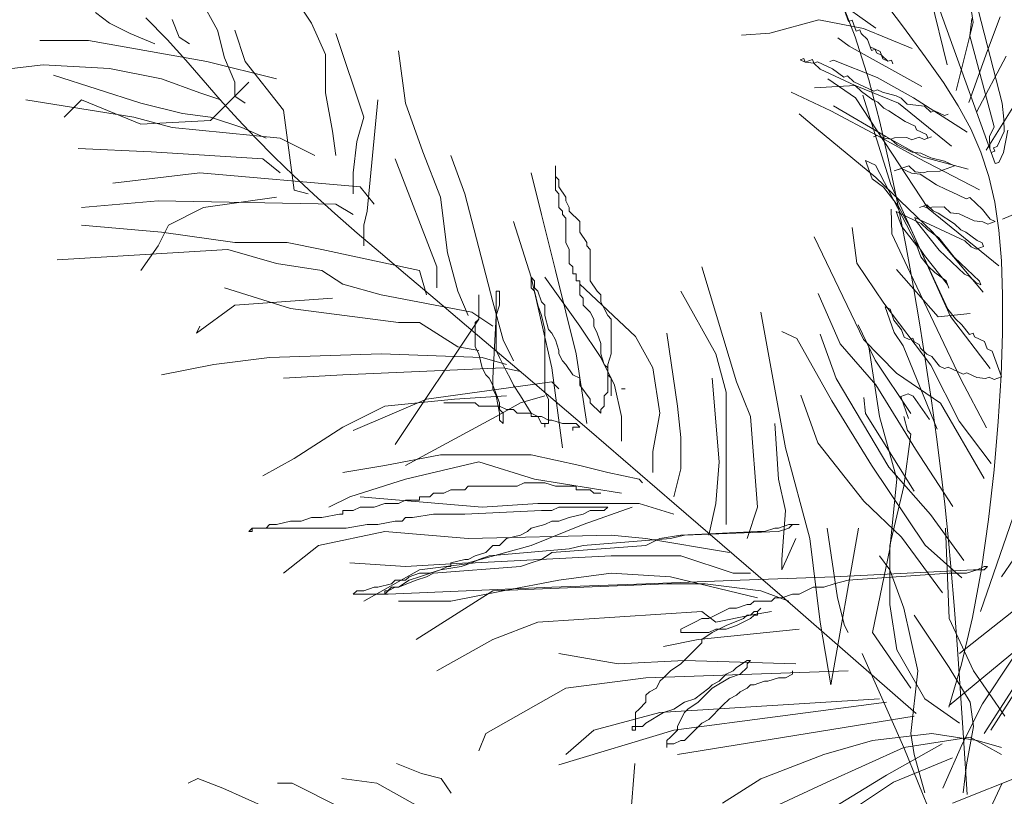
# Model space of a CAD drawing. Units: millimetres. Extents: x 595116 to 630915, y 909473 to 920225.
# Tile 72 of 134: x 629622.585 to 629629.81, y 919276.713 to 919282.412. Entities that reach past the tile are written whole.
import ezdxf

# ---------------------------------------------------------------- set-up
doc = ezdxf.new("R2010")
doc.units = ezdxf.units.MM
doc.layers.add('Dimension', color=3, linetype='Continuous', lineweight=18)
doc.layers.add('L-PLNT', color=85, linetype='Continuous', lineweight=13)
doc.styles.get("Standard").update_dxf_attribs({"font": 'arial.ttf'})
doc.dimstyles.new('ISO-25', dxfattribs={"dimtxt": 9, "dimasz": 6, "dimexe": 1.25, "dimexo": 0.625, "dimtad": 1, "dimlunit": 4, "dimtxsty": 'Standard', "dimcen": 2.5, "dimadec": 0, "dimazin": 0, "dimtfac": 1, "dimtmove": 0, "dimatfit": 3, "dimfxl": 1, "dimarcsym": 0})

# ---------------------------------------------------------------- blocks, each defined once
blk = doc.blocks.new('A$C4FB75ABC')
for p, q in [((2.7169, 3.7399), (2.6018, 4.2172)), ((2.8029, 3.5683), (2.5783, 4.1926)), ((1.2153, 3.9442), (1.2902, 3.808)), ((1.3924, 3.9442), (1.4742, 3.8217)), ((2.7679, 3.8231), (2.7507, 3.9385)), ((2.7636, 3.9026), (2.8247, 3.6653)), ((2.5777, 3.8114), (2.4796, 3.8815)), ((2.5372, 3.7949), (2.5035, 3.8821)), ((2.5794, 3.8826), (2.6314, 3.8136)), ((1.0518, 3.8421), (1.079, 3.8217)), ((1.1917, 3.7897), (1.1506, 3.8319)), ((2.5166, 3.8462), (2.5244, 3.8247)), ((2.7957, 3.7683), (2.8207, 3.834)), ((1.079, 3.8217), (1.1199, 3.8012)), ((1.2017, 3.8285), (1.2153, 3.7944)), ((1.4742, 3.8217), (1.5014, 3.7604)), ((2.4664, 3.8281), (2.3706, 3.8017)), ((2.5536, 3.8109), (2.4664, 3.8281)), ((2.5244, 3.8247), (2.5315, 3.8272)), ((2.5315, 3.8272), (2.5393, 3.8057)), ((2.6314, 3.8136), (2.6743, 3.7558)), ((2.7349, 3.6897), (2.7679, 3.8231)), ((2.7613, 3.7965), (2.7653, 3.8303)), ((1.1199, 3.8012), (1.1676, 3.7808)), ((1.2153, 3.7944), (1.2357, 3.7808)), ((1.2902, 3.808), (1.3039, 3.7536)), ((1.3243, 3.808), (1.3447, 3.7467)), ((1.5219, 3.8012), (1.5764, 3.6378)), ((2.3706, 3.8017), (2.3152, 3.798)), ((2.5255, 3.7764), (2.5034, 3.7928)), ((2.5638, 3.7106), (2.5372, 3.7949)), ((2.5393, 3.8057), (2.5464, 3.8083)), ((2.5464, 3.8083), (2.549, 3.8011)), ((2.549, 3.8011), (2.5614, 3.7893)), ((2.6486, 3.7721), (2.5536, 3.8109)), ((2.8089, 3.6191), (2.7613, 3.7965)), ((0.9428, 3.7876), (1.0382, 3.7876)), ((1.0382, 3.7876), (1.2698, 3.7467)), ((1.2284, 3.7492), (1.1917, 3.7897)), ((2.6672, 3.6978), (2.5255, 3.7764)), ((2.5614, 3.7893), (2.5665, 3.775)), ((2.5665, 3.775), (2.5763, 3.7704)), ((2.5691, 3.7678), (2.5665, 3.775)), ((1.5014, 3.7604), (1.5014, 3.6855)), ((1.6445, 3.7672), (1.6581, 3.665)), ((2.5763, 3.7704), (2.5691, 3.7678)), ((2.5763, 3.7704), (2.5789, 3.7632)), ((2.586, 3.7658), (2.5763, 3.7704)), ((2.5789, 3.7632), (2.5886, 3.7586)), ((2.5886, 3.7586), (2.586, 3.7658)), ((2.5886, 3.7586), (2.5912, 3.7515)), ((2.601, 3.7469), (2.5886, 3.7586)), ((2.6743, 3.7558), (2.7096, 3.7056)), ((2.7596, 3.6662), (2.7957, 3.7683)), ((2.7745, 3.6472), (2.8322, 3.7571)), ((0.8883, 3.7331), (0.9496, 3.7399)), ((0.9496, 3.7399), (1.079, 3.7331)), ((1.2625, 3.7099), (1.2284, 3.7492)), ((1.2698, 3.7467), (1.4061, 3.7127)), ((1.3039, 3.7536), (1.3243, 3.7059)), ((1.3447, 3.7467), (1.4197, 3.6514)), ((2.4369, 3.7526), (2.4297, 3.7501)), ((2.4297, 3.7501), (2.4394, 3.7455)), ((2.4394, 3.7455), (2.4369, 3.7526)), ((2.4538, 3.7506), (2.4394, 3.7455)), ((2.4394, 3.7455), (2.4564, 3.7435)), ((2.4564, 3.7435), (2.4538, 3.7506)), ((2.4635, 3.746), (2.4564, 3.7435)), ((2.4564, 3.7435), (2.4687, 3.7317)), ((2.4733, 3.7414), (2.4635, 3.746)), ((2.4928, 3.7323), (2.4733, 3.7414)), ((2.4948, 3.7492), (2.4876, 3.7466)), ((2.58, 3.715), (2.4948, 3.7492)), ((2.5912, 3.7515), (2.601, 3.7469)), ((2.601, 3.7469), (2.6081, 3.7494)), ((2.6081, 3.7494), (2.601, 3.7469)), ((2.6081, 3.7494), (2.6107, 3.7423)), ((2.6107, 3.7423), (2.6081, 3.7494)), ((0.97, 3.7195), (1.1403, 3.665)), ((1.079, 3.7331), (1.1812, 3.7127)), ((2.4687, 3.7317), (2.4785, 3.7271)), ((2.4785, 3.7271), (2.498, 3.7179)), ((2.5149, 3.7159), (2.4928, 3.7323)), ((2.498, 3.7179), (2.5272, 3.7041)), ((2.5221, 3.7185), (2.5149, 3.7159)), ((2.5344, 3.7067), (2.5221, 3.7185)), ((1.1812, 3.7127), (1.2562, 3.6855)), ((1.2959, 3.6716), (1.2625, 3.7099)), ((1.3515, 3.7059), (1.2766, 3.631)), ((1.3243, 3.7059), (1.3243, 3.6787)), ((2.537, 3.6995), (2.4575, 3.6952)), ((2.5376, 3.6754), (2.4836, 3.7127)), ((2.5272, 3.7041), (2.537, 3.6995)), ((2.5441, 3.7021), (2.5344, 3.7067)), ((2.537, 3.6995), (2.5493, 3.6877)), ((2.6222, 3.6653), (2.537, 3.6995)), ((2.5637, 3.6929), (2.5441, 3.7021)), ((2.5853, 3.6284), (2.5638, 3.7106)), ((2.6509, 3.6757), (2.58, 3.715)), ((2.7096, 3.7056), (2.7388, 3.6597)), ((1.2562, 3.6855), (1.297, 3.6718)), ((1.3243, 3.6787), (1.3447, 3.665)), ((1.5014, 3.6855), (1.5151, 3.6106)), ((2.4899, 3.6502), (2.4119, 3.6869)), ((2.5493, 3.6877), (2.5714, 3.6714)), ((2.6067, 3.5058), (2.5519, 3.6806)), ((2.5734, 3.6883), (2.5637, 3.6929)), ((2.5806, 3.6909), (2.5734, 3.6883)), ((2.5903, 3.6863), (2.5806, 3.6909)), ((2.617, 3.6797), (2.5903, 3.6863)), ((2.6268, 3.6751), (2.617, 3.6797)), ((2.7932, 3.5729), (2.8652, 3.6879)), ((0.9155, 3.6718), (1.1267, 3.6378)), ((1.0245, 3.6718), (0.9905, 3.6378)), ((1.1403, 3.6242), (1.0245, 3.6718)), ((1.1403, 3.665), (1.2221, 3.6446)), ((1.3299, 3.6341), (1.2959, 3.6716)), ((1.6036, 3.6718), (1.5832, 3.4539)), ((1.6581, 3.665), (1.6922, 3.5697)), ((2.5972, 3.5996), (2.4945, 3.6599)), ((2.6801, 3.4593), (2.5376, 3.6754)), ((2.5714, 3.6714), (2.5812, 3.6668)), ((2.5812, 3.6668), (2.5935, 3.655)), ((2.7255, 3.5809), (2.6222, 3.6653)), ((2.6391, 3.6633), (2.6268, 3.6751)), ((2.673, 3.6593), (2.6391, 3.6633)), ((2.7562, 3.6082), (2.6509, 3.6757)), ((2.6853, 3.6475), (2.673, 3.6593)), ((2.7388, 3.6597), (2.763, 3.6147)), ((2.8247, 3.6653), (2.8279, 3.634)), ((1.2221, 3.6446), (1.2766, 3.6378)), ((1.4197, 3.6514), (1.4401, 3.4948)), ((2.4618, 3.6157), (2.4274, 3.6439)), ((2.5803, 3.6016), (2.4899, 3.6502)), ((2.5935, 3.655), (2.6032, 3.6504)), ((2.6032, 3.6504), (2.6351, 3.6295)), ((2.6925, 3.6501), (2.6853, 3.6475)), ((2.7022, 3.6455), (2.6925, 3.6501)), ((2.712, 3.6409), (2.7022, 3.6455)), ((2.7192, 3.6435), (2.712, 3.6409)), ((1.1267, 3.6378), (1.2017, 3.6174)), ((1.2766, 3.631), (1.1403, 3.6242)), ((1.2766, 3.6378), (1.3379, 3.6174)), ((1.365, 3.5971), (1.3299, 3.6341)), ((1.5764, 3.6378), (1.5627, 3.5901)), ((2.6037, 3.5475), (2.5853, 3.6284)), ((2.6351, 3.6295), (2.6448, 3.6249)), ((2.6448, 3.6249), (2.6546, 3.6203)), ((2.6546, 3.6203), (2.6572, 3.6131)), ((2.8279, 3.634), (2.8285, 3.6099)), ((1.2017, 3.6174), (1.4129, 3.5969)), ((1.3379, 3.6174), (1.3856, 3.5969)), ((1.5151, 3.6106), (1.5219, 3.5629)), ((2.5774, 3.5196), (2.4618, 3.6157)), ((2.5803, 3.6016), (2.5731, 3.5991)), ((2.5731, 3.5991), (2.5803, 3.6016)), ((2.5901, 3.597), (2.5803, 3.6016)), ((2.5803, 3.6016), (2.5901, 3.597)), ((2.6609, 3.5577), (2.5803, 3.6016)), ((2.6572, 3.6131), (2.6669, 3.6085)), ((2.6669, 3.6085), (2.6767, 3.6039)), ((2.6767, 3.6039), (2.6793, 3.5967)), ((2.763, 3.6147), (2.7827, 3.5691)), ((2.7998, 3.5996), (2.8089, 3.6191)), ((2.8285, 3.6099), (2.8193, 3.5904)), ((2.8356, 3.6125), (2.827, 3.5688)), ((1.4014, 3.5604), (1.365, 3.5971)), ((1.4129, 3.5969), (1.481, 3.5629)), ((1.5627, 3.5901), (1.5559, 3.5288)), ((2.5972, 3.5996), (2.5901, 3.597)), ((2.5901, 3.597), (2.607, 3.595)), ((2.607, 3.595), (2.5972, 3.5996)), ((2.6681, 3.5603), (2.5972, 3.5996)), ((2.6142, 3.5976), (2.607, 3.595)), ((2.607, 3.595), (2.6193, 3.5833)), ((2.6383, 3.5982), (2.6142, 3.5976)), ((2.6193, 3.5833), (2.6486, 3.5695)), ((2.648, 3.5936), (2.6383, 3.5982)), ((2.6623, 3.5987), (2.648, 3.5936)), ((2.6721, 3.5942), (2.6623, 3.5987)), ((2.6864, 3.5993), (2.6721, 3.5942)), ((2.6793, 3.5967), (2.6864, 3.5993)), ((2.8003, 3.5755), (2.7998, 3.5996)), ((2.8193, 3.5904), (2.8147, 3.5806)), ((1.0177, 3.5765), (1.1608, 3.5697)), ((1.1608, 3.5697), (1.3788, 3.5561)), ((1.6922, 3.5697), (1.7263, 3.4812)), ((1.7467, 3.5629), (1.7739, 3.488)), ((2.6486, 3.5695), (2.6655, 3.5675)), ((2.6655, 3.5675), (2.685, 3.5583)), ((2.7827, 3.5691), (2.7983, 3.5216)), ((2.8107, 3.5468), (2.8003, 3.5755)), ((2.8101, 3.5709), (2.8029, 3.5683)), ((2.8147, 3.5806), (2.8075, 3.578)), ((2.8075, 3.578), (2.8101, 3.5709)), ((2.827, 3.5688), (2.8224, 3.5591)), ((1.3788, 3.5561), (1.4129, 3.5288)), ((1.4393, 3.5237), (1.4014, 3.5604)), ((1.6377, 3.5561), (1.7194, 3.345)), ((1.9511, 3.4948), (1.9511, 3.5425)), ((1.9511, 3.5425), (1.9511, 3.522)), ((2.5671, 3.5483), (2.5573, 3.5529)), ((2.5573, 3.5529), (2.5703, 3.517)), ((2.5769, 3.5437), (2.5671, 3.5483)), ((2.6552, 3.3935), (2.5769, 3.5437)), ((2.6204, 3.467), (2.6037, 3.5475)), ((2.642, 3.5428), (2.6133, 3.5325)), ((2.6543, 3.531), (2.642, 3.5428)), ((2.7805, 3.4954), (2.6609, 3.5577)), ((2.7579, 3.5359), (2.6681, 3.5603)), ((2.685, 3.5583), (2.7117, 3.5517)), ((2.7312, 3.5425), (2.7025, 3.5321)), ((2.7117, 3.5517), (2.7214, 3.5471)), ((2.7214, 3.5471), (2.7312, 3.5425)), ((2.8178, 3.5493), (2.8107, 3.5468)), ((2.8224, 3.5591), (2.8178, 3.5493)), ((1.0858, 3.5084), (1.2562, 3.5288)), ((1.2562, 3.5288), (1.5696, 3.5016)), ((1.4788, 3.4868), (1.4393, 3.5237)), ((1.5559, 3.5288), (1.5559, 3.488)), ((1.9034, 3.5288), (1.9238, 3.4471)), ((2.6133, 3.5325), (2.6276, 3.5376)), ((2.6276, 3.5376), (2.6471, 3.5284)), ((2.6471, 3.5284), (2.6641, 3.5264)), ((2.6712, 3.529), (2.6543, 3.531)), ((2.6641, 3.5264), (2.6959, 3.5055)), ((2.6784, 3.5316), (2.6712, 3.529)), ((2.7025, 3.5321), (2.6784, 3.5316)), ((1.9511, 3.522), (1.9579, 3.5152)), ((1.9579, 3.5152), (1.9579, 3.5016)), ((2.5703, 3.517), (2.5924, 3.5006)), ((2.6885, 3.4136), (2.5774, 3.5196)), ((2.7237, 3.248), (2.6067, 3.5058)), ((2.6959, 3.5055), (2.7154, 3.4963)), ((2.7983, 3.5216), (2.81, 3.4712)), ((1.4401, 3.4948), (1.4674, 3.488)), ((1.5201, 3.4494), (1.4788, 3.4868)), ((1.5696, 3.5016), (1.5968, 3.4676)), ((1.7739, 3.488), (1.8285, 3.2769)), ((1.9579, 3.488), (1.9511, 3.4948)), ((1.9579, 3.5016), (1.9715, 3.4812)), ((1.9579, 3.4608), (1.9579, 3.488)), ((2.5924, 3.5006), (2.6222, 3.4627)), ((2.7154, 3.4963), (2.7252, 3.4917)), ((2.7252, 3.4917), (2.7544, 3.4779)), ((2.8253, 3.4385), (2.9518, 3.4922)), ((1.0245, 3.4608), (1.1744, 3.4744)), ((1.1744, 3.4744), (1.5219, 3.4676)), ((1.4061, 3.4812), (1.263, 3.4608)), ((1.5219, 3.4676), (1.5559, 3.4471)), ((1.7263, 3.4812), (1.7399, 3.3722)), ((1.9715, 3.4812), (1.9715, 3.4744)), ((1.9715, 3.4744), (1.9783, 3.4608)), ((2.636, 3.3873), (2.6204, 3.467)), ((2.6632, 3.4613), (2.6776, 3.4664)), ((2.6776, 3.4664), (2.6899, 3.4547)), ((2.7544, 3.4779), (2.7616, 3.4805)), ((2.7616, 3.4805), (2.774, 3.4687)), ((2.774, 3.4687), (2.7863, 3.4569)), ((2.81, 3.4712), (2.8183, 3.4166)), ((1.263, 3.4608), (1.1949, 3.4267)), ((1.5633, 3.4112), (1.5201, 3.4494)), ((1.5832, 3.4539), (1.5764, 3.4267)), ((1.9238, 3.4471), (1.9511, 3.3382)), ((1.9647, 3.4539), (1.9579, 3.4608)), ((1.9647, 3.4471), (1.9647, 3.4539)), ((1.9715, 3.4403), (1.9647, 3.4471)), ((1.9783, 3.4608), (1.9783, 3.4539)), ((1.9783, 3.4539), (1.9988, 3.4335)), ((2.609, 3.4093), (2.6078, 3.4576)), ((2.6566, 3.4346), (2.6176, 3.453)), ((2.6176, 3.453), (2.6279, 3.4243)), ((2.6222, 3.4627), (2.6449, 3.4222)), ((2.6704, 3.4639), (2.6632, 3.4613)), ((2.6801, 3.4593), (2.6704, 3.4639)), ((2.6873, 3.4618), (2.6801, 3.4593)), ((2.8178, 3.3467), (2.6801, 3.4593)), ((2.7114, 3.4624), (2.6873, 3.4618)), ((2.6899, 3.4547), (2.6996, 3.4501)), ((2.6996, 3.4501), (2.7315, 3.4291)), ((2.7237, 3.4506), (2.7114, 3.4624)), ((2.7407, 3.4486), (2.7237, 3.4506)), ((2.7699, 3.4348), (2.7407, 3.4486)), ((2.7863, 3.4569), (2.8012, 3.438)), ((1.0245, 3.4267), (1.1812, 3.4131)), ((1.1949, 3.4267), (1.1744, 3.3858)), ((1.5764, 3.4267), (1.5764, 3.3858)), ((1.8693, 3.4335), (1.9034, 3.3246)), ((1.9715, 3.3927), (1.9715, 3.4403)), ((1.9988, 3.4335), (1.9988, 3.4131)), ((2.6638, 3.4372), (2.654, 3.4418)), ((2.654, 3.4418), (2.6566, 3.4346)), ((2.6566, 3.4346), (2.6664, 3.43)), ((2.6865, 3.3967), (2.6566, 3.4346)), ((2.693, 3.4234), (2.6638, 3.4372)), ((2.6664, 3.43), (2.6787, 3.4182)), ((2.7315, 3.4291), (2.7438, 3.4173)), ((2.7869, 3.4328), (2.7699, 3.4348)), ((2.7966, 3.4282), (2.7869, 3.4328)), ((2.811, 3.4334), (2.7966, 3.4282)), ((2.8012, 3.438), (2.811, 3.4334)), ((1.1812, 3.4131), (1.3243, 3.3927)), ((1.6088, 3.3721), (1.5633, 3.4112)), ((1.9988, 3.4131), (2.0124, 3.3927)), ((2.5404, 3.3522), (2.5315, 3.422)), ((2.6446, 3.333), (2.609, 3.4093)), ((2.6279, 3.4243), (2.6578, 3.3864)), ((2.6449, 3.4222), (2.7186, 3.2624)), ((2.6787, 3.4182), (2.7008, 3.4019)), ((2.7877, 3.2953), (2.6885, 3.4136)), ((2.7028, 3.4188), (2.693, 3.4234)), ((2.7223, 3.4096), (2.7028, 3.4188)), ((2.7516, 3.3958), (2.7223, 3.4096)), ((2.7438, 3.4173), (2.7536, 3.4127)), ((2.7536, 3.4127), (2.7757, 3.3964)), ((2.8183, 3.4166), (2.8233, 3.3565)), ((1.3243, 3.3927), (1.4265, 3.3927)), ((1.4265, 3.3927), (1.4946, 3.379)), ((1.9783, 3.379), (1.9715, 3.3927)), ((2.0124, 3.3927), (2.0124, 3.3858)), ((2.5536, 3.203), (2.4572, 3.4034)), ((2.6727, 3.3674), (2.6552, 3.3935)), ((2.7014, 3.3777), (2.6865, 3.3967)), ((2.7008, 3.4019), (2.7306, 3.364)), ((2.7639, 3.384), (2.7516, 3.3958)), ((2.7757, 3.3964), (2.7854, 3.3918)), ((2.7854, 3.3918), (2.788, 3.3846)), ((0.9768, 3.3586), (1.3107, 3.379)), ((1.1744, 3.3858), (1.1403, 3.3382)), ((1.3107, 3.379), (1.4061, 3.3518)), ((1.4946, 3.379), (1.6854, 3.3382)), ((1.6577, 3.3307), (1.6088, 3.3721)), ((1.7399, 3.3722), (1.7603, 3.2973)), ((1.9783, 3.3518), (1.9783, 3.379)), ((2.0124, 3.3858), (2.0192, 3.379)), ((2.0192, 3.379), (2.0192, 3.3178)), ((2.6503, 3.3086), (2.636, 3.3873)), ((2.6578, 3.3864), (2.6655, 3.3648)), ((2.7384, 3.3424), (2.7014, 3.3777)), ((2.7737, 3.3794), (2.7639, 3.384)), ((2.788, 3.3846), (2.7737, 3.3794)), ((1.4061, 3.3518), (1.4946, 3.3382)), ((1.9851, 3.345), (1.9783, 3.3518)), ((2.5929, 3.2739), (2.5404, 3.3522)), ((2.6655, 3.3648), (2.6804, 3.3459)), ((2.7174, 3.3106), (2.6727, 3.3674)), ((2.7306, 3.364), (2.743, 3.3522)), ((2.743, 3.3522), (2.7553, 3.3404)), ((2.8233, 3.3565), (2.8254, 3.2898)), ((1.4946, 3.3382), (1.5355, 3.3109)), ((1.7159, 3.2817), (1.6577, 3.3307)), ((1.6854, 3.3382), (1.699, 3.2905)), ((1.7194, 3.345), (1.7194, 3.3041)), ((1.9511, 3.3382), (1.992, 3.1748)), ((1.9851, 3.3314), (1.9851, 3.345)), ((1.992, 3.3314), (1.9851, 3.3314)), ((1.992, 3.3178), (1.992, 3.3314)), ((2.2372, 3.345), (2.3054, 3.1203)), ((2.6997, 3.2474), (2.6179, 3.3396)), ((2.7435, 3.1255), (2.6446, 3.333)), ((2.6804, 3.3459), (2.6928, 3.3341)), ((2.6928, 3.3341), (2.7149, 3.3178)), ((2.7507, 3.3307), (2.7384, 3.3424)), ((2.7605, 3.3261), (2.7507, 3.3307)), ((2.7553, 3.3404), (2.78, 3.3169)), ((1.9102, 3.3178), (1.9034, 3.3246)), ((1.9034, 3.3246), (1.9034, 3.3041)), ((1.9034, 3.3246), (1.9443, 3.1475)), ((1.9102, 3.3041), (1.9102, 3.3178)), ((1.9306, 3.3246), (1.9988, 3.2292)), ((1.9988, 3.3178), (1.992, 3.3178)), ((1.9988, 3.2905), (1.9988, 3.3178)), ((2.0192, 3.3178), (2.0328, 3.2973)), ((2.7149, 3.3178), (2.72, 3.3034)), ((2.7728, 3.3143), (2.7605, 3.3261)), ((2.7826, 3.3097), (2.7728, 3.3143)), ((2.78, 3.3169), (2.7826, 3.3097)), ((1.3039, 3.3041), (1.4333, 3.2633)), ((1.5355, 3.3109), (1.6104, 3.2905)), ((1.7603, 3.2973), (1.7808, 3.2497)), ((1.8421, 3.2973), (1.8353, 3.2973)), ((1.8353, 3.2973), (1.8353, 3.2497)), ((1.8421, 3.2701), (1.8421, 3.2973)), ((1.9034, 3.3041), (1.9102, 3.2973)), ((1.917, 3.2973), (1.9102, 3.3041)), ((1.9102, 3.2973), (1.917, 3.2701)), ((1.9238, 3.2769), (1.917, 3.2973)), ((1.9988, 3.3109), (2.1078, 3.2088)), ((2.0328, 3.2973), (2.0396, 3.2905)), ((2.1963, 3.2973), (2.2645, 3.1748)), ((2.508, 3.1947), (2.4647, 3.2926)), ((2.6635, 3.2315), (2.6503, 3.3086)), ((2.72, 3.3034), (2.7174, 3.3106)), ((1.5151, 3.2837), (1.3243, 3.2701)), ((1.6104, 3.2905), (1.7876, 3.2565)), ((1.7906, 3.2188), (1.7159, 3.2817)), ((1.8012, 3.2429), (1.8012, 3.2905)), ((1.8012, 3.2905), (1.8012, 3.2429)), ((1.8285, 3.2769), (1.8489, 3.202)), ((1.9306, 3.2701), (1.9238, 3.2769)), ((2.0056, 3.2837), (1.9988, 3.2905)), ((2.0056, 3.2701), (2.0056, 3.2837)), ((2.0396, 3.2905), (2.0396, 3.2769)), ((2.0396, 3.2769), (2.0465, 3.2633)), ((2.685, 3.153), (2.5929, 3.2739)), ((2.8254, 3.2898), (2.825, 3.2153)), ((1.3243, 3.2701), (1.2494, 3.2156)), ((1.4333, 3.2633), (1.6445, 3.236)), ((1.7876, 3.2565), (1.8285, 3.2292)), ((1.8353, 3.2497), (1.8421, 3.2701)), ((1.917, 3.2701), (1.9238, 3.2497)), ((1.9306, 3.2497), (1.9306, 3.2701)), ((2.0192, 3.2565), (2.0056, 3.2701)), ((2.026, 3.2429), (2.0192, 3.2565)), ((2.0465, 3.2633), (2.0533, 3.2497)), ((2.353, 3.2565), (2.4007, 2.9909)), ((2.6053, 3.2621), (2.5955, 3.2667)), ((2.5955, 3.2667), (2.6136, 3.2165)), ((2.613, 3.2406), (2.6053, 3.2621)), ((2.7622, 3.2537), (2.6997, 3.2474)), ((2.7186, 3.2624), (2.7335, 3.2434)), ((1.8012, 3.2429), (1.6377, 2.9977)), ((1.6445, 3.236), (1.6854, 3.236)), ((1.6854, 3.236), (1.7603, 3.1884)), ((1.7944, 3.236), (1.8012, 3.2429)), ((1.7944, 3.1884), (1.7944, 3.236)), ((1.8353, 3.2497), (1.8285, 3.1271)), ((1.8353, 3.1816), (1.8353, 3.2497)), ((1.9238, 3.2497), (1.9306, 3.2224)), ((1.9375, 3.2224), (1.9306, 3.2497)), ((2.026, 3.2292), (2.026, 3.2429)), ((2.0533, 3.2497), (2.0601, 3.2429)), ((2.0601, 3.2429), (2.0601, 3.1748)), ((2.6279, 3.2216), (2.613, 3.2406)), ((2.8009, 3.1461), (2.7237, 3.248)), ((2.7335, 3.2434), (2.7458, 3.2316)), ((1.2494, 3.2156), (1.2562, 3.2292)), ((1.8887, 3.1355), (1.7906, 3.2188)), ((1.9306, 3.2224), (1.9306, 3.0999)), ((1.9443, 3.2156), (1.9375, 3.2224)), ((1.9511, 3.202), (1.9443, 3.2156)), ((1.9988, 3.2292), (2.0396, 3.1679)), ((2.0328, 3.2156), (2.026, 3.2292)), ((2.0396, 3.1952), (2.0328, 3.2156)), ((2.1691, 3.2156), (2.1895, 3.0726)), ((2.4234, 3.2048), (2.3941, 3.2186)), ((2.5763, 3.1625), (2.5433, 3.2317)), ((2.6136, 3.2165), (2.6311, 3.1904)), ((2.6331, 3.2073), (2.6279, 3.2216)), ((2.6754, 3.1561), (2.6635, 3.2315)), ((2.7458, 3.2316), (2.7608, 3.2127)), ((2.7608, 3.2127), (2.7679, 3.2153)), ((2.7679, 3.2153), (2.7705, 3.2081)), ((2.825, 3.2153), (2.8223, 3.1323)), ((1.8489, 3.202), (1.8693, 3.1611)), ((1.9579, 3.1816), (1.9511, 3.202)), ((2.1078, 3.2088), (2.1418, 3.1475)), ((2.4914, 3.0833), (2.4234, 3.2048)), ((2.5, 3.127), (2.469, 3.2131)), ((2.6179, 3.137), (2.5536, 3.203)), ((2.6428, 3.2027), (2.6331, 3.2073)), ((2.65, 3.2053), (2.6428, 3.2027)), ((2.6526, 3.1981), (2.65, 3.2053)), ((2.6624, 3.1935), (2.6526, 3.1981)), ((2.7705, 3.2081), (2.7803, 3.2035)), ((2.7803, 3.2035), (2.79, 3.1989)), ((2.79, 3.1989), (2.7952, 3.1846)), ((1.7603, 3.1884), (1.8012, 3.1816)), ((1.8012, 3.1748), (1.7944, 3.1884)), ((1.8421, 3.1679), (1.8353, 3.1816)), ((1.9579, 3.1748), (1.9579, 3.1816)), ((2.0396, 3.1748), (2.0396, 3.1952)), ((2.5774, 3.1143), (2.508, 3.1947)), ((2.5847, 3.0522), (2.5642, 3.1884)), ((2.6311, 3.1904), (2.6976, 3.0279)), ((2.6649, 3.1863), (2.6624, 3.1935)), ((2.6773, 3.1746), (2.6649, 3.1863)), ((2.7952, 3.1846), (2.8049, 3.18)), ((2.8049, 3.18), (2.823, 3.1297)), ((1.2834, 3.1543), (1.3924, 3.1679)), ((1.3924, 3.1679), (1.6104, 3.1748)), ((1.6104, 3.1748), (1.808, 3.1679)), ((1.808, 3.1475), (1.8012, 3.1748)), ((1.808, 3.1679), (1.8557, 3.1543)), ((1.8557, 3.1407), (1.8421, 3.1679)), ((1.9647, 3.1611), (1.9579, 3.1748)), ((1.9715, 3.1543), (1.9647, 3.1611)), ((1.992, 3.1748), (2.0124, 3.0386)), ((2.0465, 3.1543), (2.0396, 3.1748)), ((2.0396, 3.1679), (2.0669, 3.1135)), ((2.0601, 3.1748), (2.0533, 3.1543)), ((2.2645, 3.1748), (2.2849, 3.0999)), ((2.6463, 3.058), (2.5763, 3.1625)), ((2.687, 3.17), (2.6773, 3.1746)), ((2.7019, 3.151), (2.687, 3.17)), ((1.1812, 3.1339), (1.2834, 3.1543)), ((1.5355, 3.1339), (1.8489, 3.1475)), ((1.8148, 3.1339), (1.808, 3.1475)), ((1.8489, 3.1475), (1.883, 3.1407)), ((1.8625, 3.1271), (1.8557, 3.1407)), ((1.9443, 3.1475), (1.9647, 2.9909)), ((1.9851, 3.1339), (1.9715, 3.1543)), ((2.0533, 3.1475), (2.0465, 3.1543)), ((2.0533, 3.1543), (2.0533, 3.0999)), ((2.0533, 3.1339), (2.0533, 3.1475)), ((2.1418, 3.1475), (2.1555, 3.059)), ((2.6863, 3.0831), (2.6754, 3.1561)), ((2.7407, 3.0434), (2.685, 3.153)), ((2.7117, 3.1464), (2.7019, 3.151)), ((2.7189, 3.149), (2.7117, 3.1464)), ((2.7286, 3.1444), (2.7189, 3.149)), ((2.7481, 3.1352), (2.7286, 3.1444)), ((1.4197, 3.1271), (1.5355, 3.1339)), ((1.699, 3.0862), (1.9443, 3.1203)), ((1.8216, 3.1271), (1.8148, 3.1339)), ((1.8285, 3.1135), (1.8216, 3.1271)), ((1.8285, 3.1271), (1.8285, 3.1067)), ((1.8693, 3.1135), (1.8625, 3.1271)), ((2.0174, 3.0255), (1.8887, 3.1355)), ((1.9443, 3.1203), (1.9579, 3.1067)), ((1.9988, 3.1271), (1.9851, 3.1339)), ((1.9988, 3.1135), (1.9988, 3.1271)), ((2.0601, 3.1271), (2.0533, 3.1339)), ((2.0601, 3.093), (2.0601, 3.1271)), ((2.2577, 3.1271), (2.2713, 2.9637)), ((2.3054, 3.1203), (2.3326, 3.0522)), ((2.603, 2.9533), (2.5, 3.127)), ((2.7037, 3.0787), (2.6179, 3.137)), ((2.794, 3.0302), (2.7435, 3.1255)), ((2.7553, 3.1378), (2.7481, 3.1352)), ((2.7651, 3.1332), (2.7553, 3.1378)), ((2.7748, 3.1286), (2.7651, 3.1332)), ((2.7917, 3.1266), (2.7748, 3.1286)), ((2.7823, 2.6709), (2.9389, 3.1271)), ((2.7989, 3.1292), (2.7917, 3.1266)), ((2.8087, 3.1246), (2.7989, 3.1292)), ((2.823, 3.1297), (2.8087, 3.1246)), ((2.8223, 3.1323), (2.817, 3.0425)), ((1.8421, 3.0794), (1.8285, 3.1135)), ((1.8285, 3.1067), (1.8353, 3.093)), ((1.883, 3.093), (1.8693, 3.1135)), ((1.9306, 3.0999), (1.9375, 3.0862)), ((2.0192, 3.0862), (1.9988, 3.1135)), ((2.0533, 3.0999), (2.0465, 3.093)), ((2.0669, 3.1135), (2.0805, 3.0522)), ((2.0873, 3.1067), (2.0805, 3.1067)), ((2.2849, 3.0999), (2.2849, 2.9024)), ((2.6552, 2.9883), (2.5774, 3.1143)), ((1.5559, 3.0249), (1.699, 3.0862)), ((1.7535, 3.0862), (1.6173, 3.0726)), ((1.8557, 3.093), (1.7535, 3.0862)), ((1.8353, 3.093), (1.8421, 3.059)), ((1.9034, 3.059), (1.883, 3.093)), ((1.883, 3.0794), (1.9306, 3.093)), ((1.9375, 3.0862), (1.9375, 3.0386)), ((2.0192, 3.0794), (2.0192, 3.0862)), ((2.0465, 3.093), (2.0465, 3.0726)), ((2.4644, 3.0007), (2.4308, 3.094)), ((2.5691, 2.9573), (2.4914, 3.0833)), ((2.5571, 3.0584), (2.5539, 3.0896)), ((2.6406, 3.0965), (2.6262, 3.0913)), ((2.6262, 3.0913), (2.6417, 3.0483)), ((2.6503, 3.0919), (2.6406, 3.0965)), ((2.6827, 3.0468), (2.6503, 3.0919)), ((2.696, 3.0126), (2.6863, 3.0831)), ((1.6173, 3.0726), (1.5355, 3.0318)), ((1.7331, 3.0794), (1.7944, 3.0794)), ((1.7944, 3.0794), (1.8012, 3.0726)), ((1.8012, 3.0726), (1.8421, 3.0726)), ((1.8353, 3.0522), (1.883, 3.0794)), ((1.8421, 3.0658), (1.8421, 3.0794)), ((1.8421, 3.0726), (1.8557, 3.0658)), ((1.8489, 3.059), (1.8421, 3.0658)), ((1.8557, 3.0658), (1.8693, 3.0658)), ((1.8693, 3.0658), (1.8761, 3.059)), ((2.0396, 3.059), (2.0192, 3.0794)), ((2.0465, 3.0726), (2.0396, 3.0658)), ((2.0396, 3.0658), (2.0396, 3.059)), ((2.1895, 3.0726), (2.1963, 3.0113)), ((2.7892, 2.9311), (2.7037, 3.0787)), ((1.6581, 2.9569), (1.8353, 3.0522)), ((1.8421, 3.059), (1.8421, 3.0454)), ((1.8421, 3.0454), (1.8489, 3.0386)), ((1.8489, 3.0386), (1.8489, 3.059)), ((1.8761, 3.059), (1.9034, 3.059)), ((1.917, 3.0522), (1.9034, 3.059)), ((1.9034, 3.059), (1.9034, 3.0522)), ((1.9034, 3.0522), (1.9238, 3.0522)), ((1.9238, 3.0386), (1.917, 3.0522)), ((1.9238, 3.0522), (1.9375, 3.0454)), ((1.9375, 3.0454), (1.9443, 3.0454)), ((1.9443, 3.0454), (1.9647, 3.0386)), ((2.0805, 3.0522), (2.0805, 3.0045)), ((2.1555, 3.059), (2.1418, 2.9841)), ((2.3326, 3.0522), (2.3462, 2.8751)), ((2.6523, 2.9062), (2.5571, 3.0584)), ((2.6187, 2.9296), (2.5847, 3.0522)), ((2.6392, 3.0249), (2.6324, 3.0522)), ((2.8029, 2.9604), (2.7407, 3.0434)), ((2.817, 3.0425), (2.809, 2.948)), ((1.5355, 3.0318), (1.4401, 2.9705)), ((1.9306, 3.0386), (1.9238, 3.0386)), ((1.9375, 3.0386), (1.9306, 3.0386)), ((1.9306, 3.0386), (1.9306, 3.0318)), ((1.9306, 3.0318), (1.9306, 3.0386)), ((1.9647, 3.0386), (1.992, 3.0386)), ((1.9988, 3.0318), (1.9851, 3.0318)), ((1.9851, 3.0318), (1.9851, 3.0249)), ((1.992, 3.0386), (1.9988, 3.0318)), ((2.1835, 2.8826), (2.0174, 3.0255)), ((2.3803, 3.0386), (2.3871, 2.9296)), ((2.646, 3.0181), (2.6392, 3.0249)), ((2.1963, 3.0113), (2.1963, 2.95)), ((2.6324, 2.916), (2.646, 3.0181)), ((2.7046, 2.9452), (2.696, 3.0126)), ((2.1418, 2.9841), (2.1418, 2.9432)), ((2.4007, 2.9909), (2.4484, 2.8139)), ((2.5539, 2.887), (2.4644, 3.0007)), ((2.7278, 2.8766), (2.6552, 2.9883)), ((1.4401, 2.9705), (1.3788, 2.9364)), ((1.6173, 2.9569), (1.7263, 2.9773)), ((1.7263, 2.9773), (1.9034, 2.9773)), ((1.9034, 2.9773), (1.9988, 2.9569)), ((1.5355, 2.9432), (1.6173, 2.9569)), ((1.8012, 2.9637), (1.6581, 2.9296)), ((1.9102, 2.9296), (1.8012, 2.9637)), ((1.9988, 2.9569), (2.0533, 2.9432)), ((2.1963, 2.95), (2.1827, 2.8956)), ((2.2713, 2.9637), (2.2645, 2.882)), ((2.6741, 2.8006), (2.5691, 2.9573)), ((2.6847, 2.8611), (2.603, 2.9533)), ((2.809, 2.948), (2.7981, 2.8512)), ((1.6581, 2.9296), (1.5491, 2.8956)), ((2.0805, 2.9024), (1.9102, 2.9296)), ((2.0533, 2.9432), (2.1146, 2.9296)), ((2.1146, 2.9296), (2.1214, 2.9228)), ((2.3871, 2.9296), (2.4007, 2.8683)), ((2.6051, 2.7934), (2.6187, 2.9296)), ((2.7122, 2.8807), (2.7046, 2.9452)), ((1.7467, 2.9092), (1.7331, 2.9024)), ((1.7739, 2.9092), (1.7467, 2.9092)), ((1.7808, 2.916), (1.7739, 2.9092)), ((1.8761, 2.916), (1.7808, 2.916)), ((1.8898, 2.9228), (1.8761, 2.916)), ((1.9306, 2.9228), (1.8898, 2.9228)), ((1.9511, 2.916), (1.9306, 2.9228)), ((1.992, 2.916), (1.9511, 2.916)), ((1.992, 2.9092), (1.992, 2.916)), ((2.0192, 2.9092), (1.992, 2.9092)), ((2.026, 2.9024), (2.0192, 2.9092)), ((2.6051, 2.8002), (2.6324, 2.916)), ((1.5491, 2.8956), (1.5082, 2.8751)), ((1.5696, 2.8956), (1.808, 2.8751)), ((1.6581, 2.8888), (1.6445, 2.882)), ((1.6854, 2.8888), (1.6581, 2.8888)), ((1.6854, 2.8956), (1.6854, 2.8888)), ((1.7058, 2.8956), (1.6854, 2.8956)), ((1.7126, 2.9024), (1.7058, 2.8956)), ((1.7331, 2.9024), (1.7126, 2.9024)), ((2.0396, 2.9024), (2.026, 2.9024)), ((2.2849, 2.9024), (2.2849, 2.8411)), ((2.8231, 2.739), (2.9253, 2.8888)), ((1.5696, 2.8751), (1.5559, 2.8683)), ((1.5968, 2.8751), (1.5696, 2.8751)), ((1.6173, 2.882), (1.5968, 2.8751)), ((1.6445, 2.882), (1.6173, 2.882)), ((1.808, 2.8751), (1.917, 2.882)), ((1.917, 2.882), (2.1146, 2.882)), ((1.9443, 2.8683), (1.9579, 2.8751)), ((1.9579, 2.8751), (2.0533, 2.8751)), ((2.101, 2.8751), (2.0056, 2.8411)), ((2.0533, 2.8751), (2.0465, 2.8683)), ((2.1146, 2.882), (2.1827, 2.8615)), ((2.3943, 2.7002), (2.1835, 2.8826)), ((2.2645, 2.882), (2.2508, 2.8207)), ((2.3462, 2.8751), (2.3258, 2.8139)), ((2.6279, 2.8164), (2.5539, 2.887)), ((2.7189, 2.8171), (2.7122, 2.8807)), ((1.4742, 2.8547), (1.4537, 2.8479)), ((1.4946, 2.8547), (1.4742, 2.8547)), ((1.5287, 2.8615), (1.4946, 2.8547)), ((1.5355, 2.8615), (1.5287, 2.8615)), ((1.5559, 2.8683), (1.5355, 2.8683)), ((1.5355, 2.8683), (1.5355, 2.8615)), ((1.6513, 2.8479), (1.6581, 2.8547)), ((1.6581, 2.8547), (1.6718, 2.8547)), ((1.6718, 2.8547), (1.7126, 2.8615)), ((1.7126, 2.8615), (1.7739, 2.8615)), ((1.7739, 2.8615), (1.9238, 2.8683)), ((1.9238, 2.8683), (1.9443, 2.8683)), ((1.9783, 2.8547), (1.9579, 2.8479)), ((2.0056, 2.8615), (1.9783, 2.8547)), ((2.0192, 2.8683), (2.0056, 2.8615)), ((2.0465, 2.8683), (2.0192, 2.8683)), ((2.4007, 2.8683), (2.3939, 2.773)), ((2.7496, 2.771), (2.6847, 2.8611)), ((2.7981, 2.8512), (2.784, 2.7542)), ((1.3515, 2.8275), (1.3584, 2.8343)), ((1.3856, 2.8343), (1.3584, 2.8343)), ((1.3584, 2.8343), (1.3584, 2.8275)), ((1.3584, 2.8343), (1.5423, 2.8343)), ((1.3924, 2.8411), (1.3856, 2.8343)), ((1.4061, 2.8411), (1.3924, 2.8411)), ((1.4333, 2.8479), (1.4061, 2.8411)), ((1.4537, 2.8479), (1.4333, 2.8479)), ((1.5423, 2.8343), (1.5832, 2.8411)), ((1.5832, 2.8411), (1.6036, 2.8411)), ((1.6036, 2.8411), (1.6377, 2.8479)), ((1.6377, 2.8479), (1.6513, 2.8479)), ((1.9034, 2.8343), (1.8966, 2.8275)), ((1.9306, 2.8411), (1.9034, 2.8343)), ((2.0056, 2.8411), (1.9034, 2.8002)), ((1.9443, 2.8479), (1.9306, 2.8411)), ((1.9579, 2.8479), (1.9443, 2.8479)), ((2.3599, 2.8275), (2.3803, 2.8343)), ((2.3803, 2.8343), (2.3871, 2.8343)), ((2.3871, 2.8343), (2.4075, 2.8411)), ((2.4075, 2.8343), (2.3871, 2.8275)), ((2.4075, 2.8411), (2.428, 2.8411)), ((2.4144, 2.8411), (2.4075, 2.8343)), ((2.428, 2.8411), (2.4144, 2.8411)), ((2.4825, 2.8343), (2.5029, 2.6981)), ((2.4893, 2.5279), (2.5438, 2.8343)), ((2.7209, 2.6572), (2.7141, 2.8343)), ((1.3584, 2.8275), (1.3515, 2.8275)), ((1.4878, 2.8002), (1.6173, 2.8275)), ((1.6173, 2.8275), (1.7808, 2.8139)), ((1.7808, 2.8139), (2.0601, 2.8207)), ((1.8557, 2.8139), (1.8421, 2.8002)), ((1.883, 2.8207), (1.8557, 2.8139)), ((1.8966, 2.8275), (1.883, 2.8207)), ((2.1759, 2.8139), (2.0056, 2.8002)), ((2.0601, 2.8207), (2.1282, 2.8139)), ((2.1282, 2.8002), (2.1555, 2.8139)), ((2.1282, 2.8139), (2.2917, 2.7866)), ((2.1555, 2.8139), (2.1963, 2.8207)), ((2.2032, 2.8207), (2.1759, 2.8139)), ((2.1963, 2.8207), (2.3462, 2.8275)), ((2.3871, 2.8275), (2.2032, 2.8207)), ((2.3462, 2.8275), (2.3599, 2.8275)), ((2.3939, 2.7526), (2.4212, 2.8139)), ((2.4484, 2.8139), (2.4689, 2.6504)), ((2.7077, 2.7073), (2.6279, 2.8164)), ((2.7251, 2.7519), (2.7189, 2.8171)), ((1.4197, 2.7458), (1.4878, 2.8002)), ((1.9034, 2.8002), (1.7808, 2.7662)), ((1.8285, 2.8002), (1.8148, 2.7866)), ((1.9783, 2.7934), (1.8216, 2.7798)), ((1.8421, 2.8002), (1.8285, 2.8002)), ((1.9443, 2.7866), (2.1282, 2.8002)), ((2.0056, 2.8002), (1.9783, 2.7934)), ((2.5711, 2.63), (2.6051, 2.7934)), ((2.6051, 2.6845), (2.6051, 2.8002)), ((2.7456, 2.7371), (2.6741, 2.8006)), ((1.7739, 2.773), (1.7467, 2.7662)), ((1.7808, 2.773), (1.7739, 2.773)), ((1.7944, 2.7798), (1.7808, 2.773)), ((1.8012, 2.773), (1.7876, 2.7662)), ((1.8148, 2.7866), (1.7944, 2.7798)), ((1.7944, 2.7662), (2.0601, 2.7798)), ((1.8216, 2.7798), (1.8012, 2.773)), ((1.9034, 2.7662), (1.9238, 2.773)), ((1.9238, 2.773), (1.9443, 2.7866)), ((2.0601, 2.7798), (2.1078, 2.7798)), ((2.1078, 2.7798), (2.1963, 2.7798)), ((2.1963, 2.7798), (2.2985, 2.7458)), ((2.3939, 2.773), (2.3939, 2.7526)), ((2.6051, 2.7526), (2.5847, 2.7798)), ((1.6581, 2.7594), (1.5491, 2.7662)), ((1.7808, 2.7662), (1.6581, 2.7594)), ((1.6854, 2.7526), (1.7944, 2.7662)), ((1.7126, 2.7458), (1.883, 2.7594)), ((1.7399, 2.7594), (1.7263, 2.7526)), ((1.7671, 2.7594), (1.7263, 2.7526)), ((1.7467, 2.7594), (1.7399, 2.7594)), ((1.7467, 2.7662), (1.7467, 2.7594)), ((1.7876, 2.7662), (1.7671, 2.7594)), ((1.883, 2.7594), (1.9034, 2.7662)), ((2.784, 2.7542), (2.7664, 2.6591)), ((2.7891, 2.7594), (2.7754, 2.7526)), ((2.7891, 2.7526), (2.7959, 2.7594)), ((2.7959, 2.7594), (2.7891, 2.7594)), ((1.5764, 2.6913), (1.6854, 2.7526)), ((1.6649, 2.739), (1.6581, 2.7321)), ((1.6854, 2.7458), (1.6649, 2.739)), ((1.6854, 2.739), (1.6649, 2.7321)), ((1.6786, 2.7321), (1.699, 2.739)), ((1.7263, 2.7526), (1.6854, 2.739)), ((1.7058, 2.7458), (1.6854, 2.7458)), ((1.699, 2.739), (1.7126, 2.7458)), ((1.7263, 2.7526), (1.7058, 2.7458)), ((2.0601, 2.7458), (1.9579, 2.7321)), ((2.1759, 2.739), (2.0601, 2.7458)), ((2.3462, 2.6981), (2.1759, 2.739)), ((2.2985, 2.7458), (2.3326, 2.7458)), ((2.3122, 2.7321), (2.4961, 2.739)), ((2.4961, 2.739), (2.7686, 2.7526)), ((2.7209, 2.7458), (2.5234, 2.7321)), ((2.6324, 2.6777), (2.6051, 2.7526)), ((2.755, 2.7458), (2.7209, 2.7458)), ((2.7309, 2.6826), (2.7251, 2.7519)), ((2.7754, 2.7526), (2.755, 2.7458)), ((2.7686, 2.7526), (2.7891, 2.7526)), ((1.5968, 2.7185), (1.5764, 2.7117)), ((1.6036, 2.7185), (1.5968, 2.7185)), ((1.6309, 2.7253), (1.6036, 2.7185)), ((1.6309, 2.7185), (1.6173, 2.7049)), ((1.6241, 2.7117), (1.6377, 2.7185)), ((1.6241, 2.7049), (1.9443, 2.7185)), ((1.6377, 2.7321), (1.6309, 2.7253)), ((1.6445, 2.7185), (1.6309, 2.7185)), ((1.6581, 2.7321), (1.6377, 2.7321)), ((1.6377, 2.7185), (1.6445, 2.7185)), ((1.6649, 2.7321), (1.6445, 2.7185)), ((1.6445, 2.7185), (1.6786, 2.7321)), ((1.8285, 2.7117), (2.1691, 2.7253)), ((1.9579, 2.7321), (1.8489, 2.7117)), ((1.9443, 2.7185), (2.1282, 2.7253)), ((2.1282, 2.7253), (2.3122, 2.7321)), ((2.1691, 2.7253), (2.244, 2.7253)), ((2.244, 2.7253), (2.353, 2.7117)), ((2.4552, 2.7185), (2.428, 2.7049)), ((2.4757, 2.7185), (2.4552, 2.7185)), ((2.4961, 2.7253), (2.4757, 2.7185)), ((2.5234, 2.7321), (2.4961, 2.7253)), ((2.7414, 2.5891), (2.9049, 2.7185)), ((1.5627, 2.7117), (1.5559, 2.7049)), ((1.5559, 2.7049), (1.6241, 2.7049)), ((1.5764, 2.7117), (1.5627, 2.7117)), ((1.6173, 2.7049), (1.6173, 2.7117)), ((1.6173, 2.7117), (1.6241, 2.7117)), ((1.6786, 2.6164), (1.8285, 2.7117)), ((1.8489, 2.7117), (1.7467, 2.6913)), ((2.353, 2.7117), (2.4075, 2.6913)), ((2.3803, 2.6981), (2.3735, 2.6913)), ((2.3939, 2.6981), (2.3803, 2.6981)), ((2.4144, 2.7049), (2.3939, 2.6981)), ((2.6566, 2.472), (2.3943, 2.7002)), ((2.428, 2.7049), (2.4144, 2.7049)), ((2.5029, 2.6981), (2.5166, 2.6436)), ((1.7467, 2.6913), (1.6445, 2.6913)), ((2.2917, 2.6777), (2.2508, 2.6572)), ((2.3054, 2.6777), (2.2917, 2.6777)), ((2.3258, 2.6845), (2.3054, 2.6777)), ((2.3326, 2.6845), (2.3258, 2.6845)), ((2.3394, 2.6913), (2.3326, 2.6845)), ((2.3735, 2.6913), (2.3394, 2.6913)), ((2.3462, 2.6709), (2.353, 2.6777)), ((2.353, 2.6777), (2.3462, 2.6709)), ((2.6187, 2.596), (2.6051, 2.6845)), ((2.6596, 2.5551), (2.6324, 2.6777)), ((2.7367, 2.6065), (2.7309, 2.6826)), ((1.917, 2.6504), (2.2372, 2.6709)), ((2.2372, 2.6572), (2.2236, 2.6504)), ((2.2372, 2.6709), (2.2645, 2.6504)), ((2.2508, 2.6572), (2.2372, 2.6572)), ((2.2645, 2.6504), (2.3326, 2.664)), ((2.319, 2.6572), (2.2849, 2.6436)), ((2.3054, 2.6436), (2.3326, 2.6572)), ((2.3258, 2.664), (2.319, 2.6572)), ((2.3326, 2.664), (2.3258, 2.664)), ((2.3394, 2.6709), (2.3326, 2.664)), ((2.3326, 2.664), (2.3735, 2.6709)), ((2.3326, 2.6572), (2.3394, 2.664)), ((2.3462, 2.6709), (2.3394, 2.6709)), ((2.3394, 2.664), (2.3462, 2.664)), ((2.3462, 2.664), (2.3462, 2.6709)), ((2.6528, 2.664), (2.7209, 2.5619)), ((2.7209, 2.487), (2.9253, 2.6572)), ((2.7686, 2.5551), (2.7209, 2.6572)), ((2.7664, 2.6591), (2.7451, 2.5683)), ((1.8285, 2.6164), (1.917, 2.6504)), ((2.2236, 2.6504), (2.1963, 2.6368)), ((2.2849, 2.6436), (2.2577, 2.63)), ((2.2849, 2.6368), (2.3054, 2.6436)), ((2.4689, 2.6504), (2.4893, 2.5279)), ((2.5166, 2.6436), (2.5234, 2.63)), ((2.1963, 2.6368), (2.1963, 2.63)), ((2.1963, 2.63), (2.2508, 2.63)), ((2.428, 2.6368), (2.2304, 2.6164)), ((2.2577, 2.63), (2.2372, 2.6164)), ((2.2508, 2.63), (2.2645, 2.6368)), ((2.2645, 2.6368), (2.2849, 2.6368)), ((2.646, 2.5211), (2.5711, 2.63)), ((1.7194, 2.5551), (1.8285, 2.6164)), ((2.2304, 2.6164), (2.1623, 2.6028)), ((2.2372, 2.6096), (2.2236, 2.596)), ((2.2372, 2.6164), (2.2372, 2.6096)), ((2.7426, 2.5213), (2.7367, 2.6065)), ((2.0737, 2.5687), (1.9579, 2.5891)), ((2.21, 2.5823), (2.1963, 2.5687)), ((2.2236, 2.596), (2.21, 2.5823)), ((2.5506, 2.5891), (2.6324, 2.4053)), ((2.6732, 2.5006), (2.6187, 2.596)), ((2.2032, 2.5755), (2.0737, 2.5687)), ((2.1963, 2.5687), (2.1759, 2.5551)), ((2.4212, 2.5687), (2.2032, 2.5755)), ((2.2985, 2.5551), (2.3054, 2.5619)), ((2.3054, 2.5619), (2.3258, 2.5755)), ((2.3258, 2.5619), (2.3122, 2.5483)), ((2.3258, 2.5755), (2.3326, 2.5755)), ((2.3326, 2.5755), (2.3258, 2.5687)), ((2.3258, 2.5687), (2.3258, 2.5619)), ((2.7451, 2.5683), (2.72, 2.484)), ((2.7209, 2.5619), (2.7618, 2.4938)), ((2.786, 2.4905), (2.8442, 2.5778)), ((2.1282, 2.5415), (1.9715, 2.5211)), ((2.5234, 2.5551), (2.1282, 2.5415)), ((2.1623, 2.5415), (2.1555, 2.5347)), ((2.1759, 2.5551), (2.1623, 2.5415)), ((2.2917, 2.5415), (2.2577, 2.5211)), ((2.2713, 2.5347), (2.2781, 2.5415)), ((2.2781, 2.5415), (2.2849, 2.5483)), ((2.2849, 2.5483), (2.2985, 2.5551)), ((2.3122, 2.5483), (2.2917, 2.5415)), ((2.3667, 2.5347), (2.3871, 2.5415)), ((2.3871, 2.5415), (2.4007, 2.5415)), ((2.4007, 2.5415), (2.4144, 2.5483)), ((2.4144, 2.5483), (2.4144, 2.5551)), ((2.646, 2.4325), (2.6596, 2.5551)), ((2.8299, 2.4666), (2.7686, 2.5551)), ((2.1555, 2.5347), (2.1487, 2.5211)), ((2.2508, 2.5211), (2.2577, 2.5279)), ((2.2577, 2.5279), (2.2713, 2.5347)), ((2.3258, 2.5211), (2.3326, 2.5279)), ((2.3326, 2.5279), (2.3394, 2.5279)), ((2.3394, 2.5279), (2.3599, 2.5347)), ((2.3599, 2.5347), (2.3667, 2.5347)), ((2.7891, 2.4325), (2.8504, 2.5279)), ((2.8027, 2.4393), (2.864, 2.5347)), ((1.9715, 2.5211), (1.8148, 2.4325)), ((2.135, 2.5142), (2.1282, 2.5074)), ((2.1282, 2.5074), (2.1282, 2.4938)), ((2.1487, 2.5211), (2.135, 2.5142)), ((2.2236, 2.5006), (2.2508, 2.5211)), ((2.244, 2.5074), (2.2304, 2.4938)), ((2.2577, 2.5211), (2.244, 2.5074)), ((2.2917, 2.5006), (2.3054, 2.5074)), ((2.3054, 2.5074), (2.3122, 2.5142)), ((2.3122, 2.5142), (2.3258, 2.5211)), ((2.7489, 2.4244), (2.7426, 2.5213)), ((2.1282, 2.4938), (2.1146, 2.4802)), ((2.5847, 2.5006), (2.1555, 2.4734)), ((2.1827, 2.4802), (2.2032, 2.4938)), ((2.5983, 2.4938), (2.1827, 2.4393)), ((2.2032, 2.4938), (2.2236, 2.5006)), ((2.2304, 2.4938), (2.21, 2.4802)), ((2.2508, 2.4598), (2.2781, 2.487)), ((2.2781, 2.487), (2.2917, 2.5006)), ((2.7414, 2.453), (2.6732, 2.5006)), ((2.7471, 2.4129), (2.786, 2.4905)), ((2.7618, 2.4938), (2.7686, 2.4461)), ((2.1555, 2.4734), (2.026, 2.4393)), ((2.1146, 2.4802), (2.1078, 2.4734)), ((2.1078, 2.4734), (2.1078, 2.4461)), ((2.1282, 2.453), (2.1623, 2.4734)), ((2.1623, 2.4734), (2.1827, 2.4802)), ((2.6528, 2.4666), (2.1895, 2.3917)), ((2.2032, 2.4734), (2.1963, 2.4598)), ((2.21, 2.4802), (2.2032, 2.4734)), ((2.1078, 2.4461), (2.101, 2.4461)), ((2.101, 2.4461), (2.101, 2.4393)), ((2.1078, 2.4393), (2.1078, 2.4461)), ((2.1078, 2.4461), (2.1214, 2.4461)), ((2.1214, 2.4461), (2.1282, 2.453)), ((2.1963, 2.4598), (2.1895, 2.4461)), ((2.1895, 2.4461), (2.1895, 2.4393)), ((2.2236, 2.4393), (2.2372, 2.453)), ((2.2372, 2.453), (2.2508, 2.4598)), ((2.7686, 2.4461), (2.755, 2.3712)), ((1.8148, 2.4325), (1.8012, 2.3985)), ((2.1827, 2.4393), (1.9579, 2.3712)), ((2.026, 2.4393), (1.9715, 2.3917)), ((2.101, 2.4393), (2.1078, 2.4393)), ((2.1759, 2.4257), (2.1691, 2.4189)), ((2.1895, 2.4393), (2.1759, 2.4257)), ((2.2032, 2.4189), (2.2236, 2.4393)), ((2.5711, 2.4189), (2.6869, 2.4325)), ((2.6324, 2.4053), (2.7618, 2.4257)), ((2.6528, 2.3917), (2.646, 2.4325)), ((2.6869, 2.4325), (2.7754, 2.4189)), ((2.7618, 2.4257), (2.8231, 2.3917)), ((2.1691, 2.4189), (2.1691, 2.4053)), ((2.1691, 2.4053), (2.1691, 2.4121)), ((2.1691, 2.4121), (2.1827, 2.4121)), ((2.1827, 2.4121), (2.1963, 2.4189)), ((2.1963, 2.4189), (2.2032, 2.4189)), ((2.4757, 2.3917), (2.5711, 2.4189)), ((2.7073, 2.4121), (2.5983, 2.3508)), ((2.7083, 2.3255), (2.7471, 2.4129)), ((2.7559, 2.3132), (2.7489, 2.4244)), ((2.7754, 2.4189), (2.8231, 2.4053)), ((2.353, 2.344), (2.4757, 2.3917)), ((2.4825, 2.3372), (2.6324, 2.4053)), ((2.6324, 2.4053), (2.7073, 2.2214)), ((2.6732, 2.3168), (2.6528, 2.3917)), ((1.6891, 2.3546), (1.6405, 2.3741)), ((2.1065, 2.3741), (2.087, 2.1315)), ((2.7277, 2.3849), (2.6119, 2.3372)), ((2.755, 2.3712), (2.7482, 2.3168)), ((1.7279, 2.3449), (1.6891, 2.3546)), ((2.5983, 2.3508), (2.4757, 2.2759)), ((2.7277, 2.2964), (2.8733, 2.3546)), ((1.2522, 2.3449), (1.2328, 2.3352)), ((1.3008, 2.3255), (1.2522, 2.3449)), ((1.4367, 2.3352), (1.4075, 2.3352)), ((1.5337, 2.2867), (1.4367, 2.3352)), ((1.6017, 2.3352), (1.5337, 2.3449)), ((1.6891, 2.2867), (1.6017, 2.3352)), ((1.7473, 2.3158), (1.7279, 2.3449)), ((2.2781, 2.2963), (2.353, 2.344)), ((2.3054, 2.2555), (2.4825, 2.3372)), ((2.6119, 2.3372), (2.5302, 2.2827)), ((2.8248, 2.3352), (2.7471, 2.1703)), ((1.3881, 2.2867), (1.3008, 2.3255))]:
    blk.add_line(p, q)
blk = doc.blocks.new('*D216')
at = {"layer": 'Defpoints', "color": 0, "transparency": 16777216}
for p in [(629743.5408, 919411.9276), (629505.0408, 919411.8279), (629743.5408, 918832.3776)]:
    blk.add_point(p, dxfattribs=at)
at = {"layer": 'Dimension', "color": 0, "lineweight": -2, "transparency": 16777216}
for p, q in [((629743.5408, 919411.3026), (629743.5408, 918831.1276)), ((629505.0408, 919411.2029), (629505.0408, 918831.1276)), ((629511.0408, 918832.3776), (629737.5408, 918832.3776))]:
    blk.add_line(p, q, dxfattribs=at)
at = {"layer": 'Dimension', "color": 0, "transparency": 16777216}
for points in [[(629511.0408, 918833.3776), (629511.0408, 918831.3776), (629505.0408, 918832.3776)], [(629737.5408, 918833.3776), (629737.5408, 918831.3776), (629743.5408, 918832.3776)]]:
    blk.add_solid(points, dxfattribs=at)
at = {"layer": 'Dimension', "color": 0, "transparency": 16777216, "insert": (629624.2908, 918837.656), "char_height": 9, "attachment_point": 5}
blk.add_mtext('19\'-10 1/2"', dxfattribs=at)

msp = doc.modelspace()

# ---------------------------------------------------------------- block references
at = {"layer": 'L-PLNT', "xscale": 3.753413438031968, "yscale": 3.753413438031968, "zscale": 3.753413438031968}
msp.add_blockref('A$C4FB75ABC', (629619.1929, 919268.043), dxfattribs=at)

# ---------------------------------------------------------------- dimensions: what is measured, and where the dimension line sits
at = {"layer": 'Dimension'}
dim = msp.add_linear_dim(base=(629743.5408, 918832.3776), p1=(629505.0408, 919411.8279), p2=(629743.5408, 919411.9276), dimstyle='ISO-25', override={"dimdec": 1, "dimlfac": 1, "dimrnd": 0, "dimzin": 1, "dimdsep": 46, "dimlunit": 4, "dimfrac": 2}, dxfattribs=at)
dim.commit()
dim.dimension.update_dxf_attribs({"geometry": '*D216', "text_midpoint": (629624.2908, 918837.656)})

doc.saveas('drawing.dxf')
